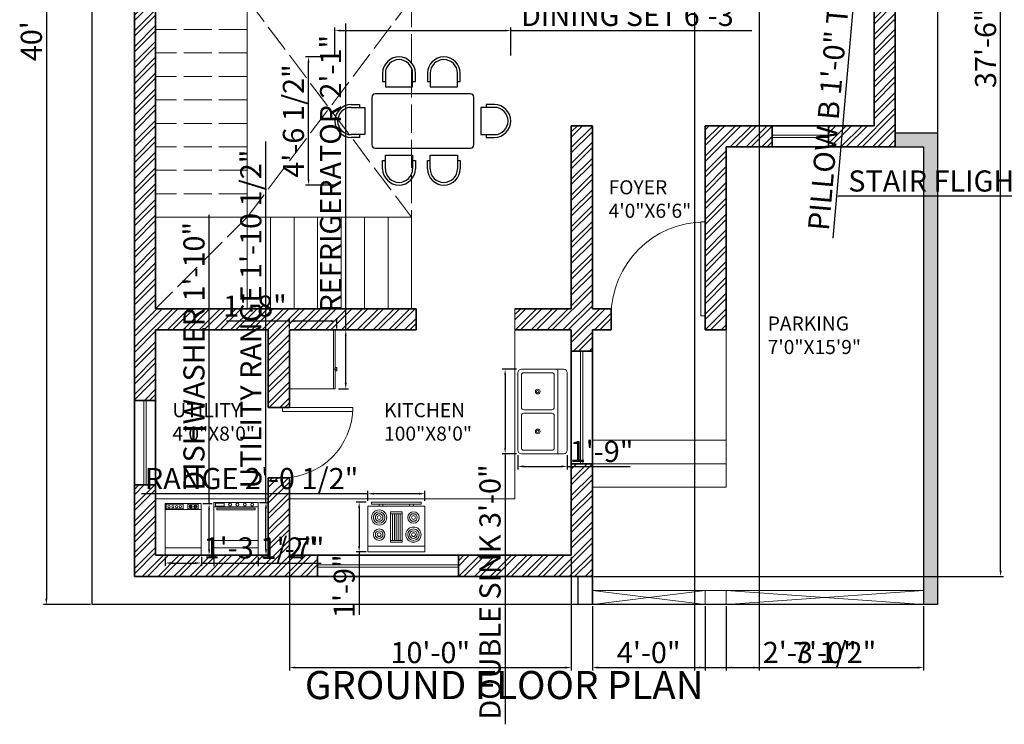
# Model space of a CAD drawing. Units: inches. Extents: x 638 to 1853, y 4393 to 5041.
# Tile 1 of 6: x 653 to 1072, y 4393 to 4693. Entities that reach past the tile are written whole.
import ezdxf

# ---------------------------------------------------------------- set-up
doc = ezdxf.new("R2010")
doc.units = ezdxf.units.IN
doc.linetypes.add('ACAD_ISO02W100', pattern=[15, 12, -3])
for name, color, linetype, lineweight in [('A-ANNO-DIMS', 2, 'Continuous', 18), ('A-ANNO-TEXT', 7, 'Continuous', 25), ('A-AREA-IDEN', 7, 'Continuous', 18), ('A-DOOR', 4, 'Continuous', 18), ('A-EQPM', 8, 'Continuous', 18), ('A-FLOR-CASE', 7, 'Continuous', 18), ('A-FLOR-FIXT', 9, 'Continuous', 18), ('A-FLOR-STRS', 7, 'Continuous', 18), ('A-FLOR-STRS-HIDN', 7, 'ACAD_ISO02W100', 18), ('A-FURN', 26, 'Continuous', 13), ('A-GLAZ', 5, 'Continuous', 18), ('A-WALL', 7, 'Continuous', 35), ('A-WALL-PATT', 251, 'Continuous', 13), ('A-WALL-PRPT', 7, 'Continuous', 25), ('A-WALL-PRPT-PATT', 141, 'Continuous', 13), ('C-PROP', 7, 'Continuous', 25), ('L-GATE', 3, 'Continuous', 18)]:
    doc.layers.add(name, color=color, linetype=linetype, lineweight=lineweight)
doc.layers.add('NOI THAT', color=42, linetype='Continuous')
doc.styles.get("Standard").update_dxf_attribs({"font": 'arial.ttf'})
doc.dimstyles.new('ISO-25', dxfattribs={"dimtxt": 9, "dimasz": 2.5, "dimexe": 1.25, "dimexo": 0.625, "dimtad": 1, "dimdec": 1, "dimlunit": 3, "dimtxsty": 'Standard', "dimcen": 2.5, "dimadec": 0, "dimazin": 0, "dimtfac": 1, "dimtdec": 1, "dimtmove": 0, "dimatfit": 3, "dimfxl": 1, "dimarcsym": 0})

# ---------------------------------------------------------------- blocks, each defined once
blk = doc.blocks.new('*U5')
for p, q in [((0, 0), (0, -6)), ((-40, 0), (-40, -6))]:
    blk.add_line(p, q)
blk.add_lwpolyline([(0, 0), (0, 40), (-1.75, 40), (-1.75, 0)], close=True)
blk.add_arc((0, 0), 40, 90, 180)
blk = doc.blocks.new('*U6')
for p, q in [((-30, 0), (-30, 6)), ((0, 0), (0, 6))]:
    blk.add_line(p, q)
blk.add_lwpolyline([(0, 0), (0, -30), (-1.75, -30), (-1.75, 0)], close=True)
blk.add_arc((0, 0), 30, 180, 270)
blk = doc.blocks.new('*D17')
at = {"layer": 'A-ANNO-DIMS', "color": 0, "lineweight": -2, "transparency": 16777216}
for p, q in [((682.72, 4924.19), (662.61, 4924.19)), ((663.86, 4921.69), (663.86, 4446.69)), ((682.72, 4444.19), (662.61, 4444.19))]:
    blk.add_line(p, q, dxfattribs=at)
at = {"layer": 'A-ANNO-DIMS', "color": 0, "transparency": 16777216}
for points in [[(663.44, 4921.69), (664.28, 4921.69), (663.86, 4924.19)], [(663.44, 4446.69), (664.28, 4446.69), (663.86, 4444.19)]]:
    blk.add_solid(points, dxfattribs=at)
at = {"layer": 'Defpoints', "color": 0, "transparency": 16777216}
for p in [(683.34, 4924.19), (663.86, 4444.19), (683.34, 4444.19)]:
    blk.add_point(p, dxfattribs=at)
at = {"layer": 'A-ANNO-DIMS', "color": 0, "transparency": 16777216, "insert": (658.64, 4684.19), "char_height": 9, "attachment_point": 5, "rotation": 90}
blk.add_mtext("40'", dxfattribs=at)
blk = doc.blocks.new('A$C3F0C2877')
at = {"layer": 'NOI THAT'}
for p, q in [((700, 1640), (700, 1520)), ((740, 1640), (740, 1440)), ((1140, 1440), (1140, 1640)), ((1180, 1520), (1180, 1640)), ((1358, 1640), (1358, 1520)), ((1398, 1640), (1398, 1440)), ((1798, 1440), (1798, 1640)), ((1838, 1520), (1838, 1640)), ((700, 1520), (740, 1520)), ((1140, 1520), (1180, 1520)), ((1358, 1520), (1398, 1520)), ((1798, 1520), (1838, 1520)), ((1988, 1340), (590, 1340)), ((740, 1440), (1140, 1440)), ((1398, 1440), (1798, 1440)), ((240, 1180), (360, 1180)), ((360, 1180), (360, 1140)), ((540, 1290), (540, 590)), ((2038, 590), (2038, 1290)), ((2339, 1180), (2219, 1180)), ((2219, 1180), (2219, 1140)), ((240, 1140), (440, 1140)), ((440, 1140), (440, 740)), ((2139, 1140), (2139, 740)), ((2339, 1140), (2139, 1140)), ((440, 740), (240, 740)), ((360, 740), (360, 700)), ((2139, 740), (2339, 740)), ((2219, 740), (2219, 700)), ((360, 700), (240, 700)), ((2219, 700), (2339, 700)), ((590, 540), (1988, 540)), ((740, 440), (1140, 440)), ((740, 240), (740, 440)), ((1140, 440), (1140, 240)), ((1398, 440), (1798, 440)), ((1398, 240), (1398, 440)), ((1798, 440), (1798, 240)), ((700, 360), (740, 360)), ((700, 240), (700, 360)), ((1140, 360), (1180, 360)), ((1180, 360), (1180, 240)), ((1358, 360), (1398, 360)), ((1358, 240), (1358, 360)), ((1798, 360), (1838, 360)), ((1838, 360), (1838, 240))]:
    blk.add_line(p, q, dxfattribs=at)
for centre, radius, start, end in [((940, 1640), 240, 0, 180), ((1598, 1640), 240, 0, 180), ((940, 1640), 200, 0, 180), ((1598, 1640), 200, 0, 180), ((590, 1290), 50, 90, 180), ((1988, 1290), 50, 0, 90), ((240, 940), 240, 90, 270), ((2339, 940), 240, 270, 90), ((240, 940), 200, 90, 270), ((2339, 940), 200, 270, 90), ((590, 590), 50, 180, 270), ((1988, 590), 50, 270, 0), ((940, 240), 240, 180, 0), ((940, 240), 200, 180, 0), ((1598, 240), 240, 180, 0), ((1598, 240), 200, 180, 0)]:
    blk.add_arc(centre, radius, start, end, dxfattribs=at)
blk = doc.blocks.new('Sink-double - 36 in top')
for p, q in [((-18, -4), (18, -4)), ((-0.75, -18.5), (-0.75, -6.5)), ((0.75, -6.5), (0.75, -18.5))]:
    blk.add_line(p, q)
for points in [[(-16.5, 0), (16.5, 0)], [(-18, -19.5), (-18, -1.5)], [(18, -1.5), (18, -19.5)], [(-16.5, -18.5), (-16.5, -6.5)], [(-15.5, -5.5), (-1.75, -5.5)], [(1.75, -5.5), (15.5, -5.5)], [(16.5, -6.5), (16.5, -18.5)], [(-1.75, -19.5), (-15.5, -19.5)], [(15.5, -19.5), (1.75, -19.5)], [(16.5, -21), (-16.5, -21)]]:
    blk.add_lwpolyline(points)
for centre, radius in [((-8.5, -12.5), 1), ((-8.5, -12.5), 0.5), ((8.5, -12.5), 1), ((8.5, -12.5), 0.5)]:
    blk.add_circle(centre, radius)
for centre, radius, start, end in [((-16.5, -1.5), 1.5, 90, 180), ((16.5, -1.5), 1.5, 0, 90), ((-15.5, -6.5), 1, 90, 180), ((-1.75, -6.5), 1, 0, 90), ((1.75, -6.5), 1, 90, 180), ((15.5, -6.5), 1, 0, 90), ((-16.5, -19.5), 1.5, 180, 270), ((-15.5, -18.5), 1, 180, 270), ((-1.75, -18.5), 1, 270, 0), ((1.75, -18.5), 1, 180, 270), ((15.5, -18.5), 1, 270, 0), ((16.5, -19.5), 1.5, 270, 0)]:
    blk.add_arc(centre, radius, start, end)
blk = doc.blocks.new('Range-Oven - 30 in top')
for p, q in [((0, -3), (30, -3)), ((12, -6), (18, -6)), ((13, -20), (13, -6)), ((14, -6), (14, -20)), ((15, -20), (15, -6)), ((16, -6), (16, -20)), ((17, -20), (17, -6)), ((18, -20), (12, -20)), ((6, -24), (6, -25)), ((8, -25), (8, -24)), ((22, -25), (22, -24)), ((24, -24), (24, -25))]:
    blk.add_line(p, q)
for points in [[(0, -24), (0, 0), (30, 0), (30, -24)], [(12, -21), (12, -5), (18, -5), (18, -21)], [(2, -26), (2, -25), (28, -25), (28, -26)]]:
    blk.add_lwpolyline(points, close=True)
for centre, radius in [((6, -9), 4), ((6, -9), 3), ((6, -9), 2), ((6, -9), 1), ((24, -9), 3), ((24, -9), 2), ((24, -9), 1), ((6, -18), 3), ((24, -18), 4), ((24, -18), 3), ((6, -18), 2), ((6, -18), 1), ((24, -18), 2), ((24, -18), 1)]:
    blk.add_circle(centre, radius)
blk = doc.blocks.new('Range-Oven - 30 in front')
for p, q in [((0, 33.00005), (30, 33.00005)), ((30, 10), (0, 10)), ((0, 5), (30, 5))]:
    blk.add_line(p, q)
for points in [[(0, 0), (0, 36.00005), (30, 36.00005), (30, 0)], [(1, 33.50005), (1, 35.50005), (7, 35.50005), (7, 33.50005)], [(2, 31.00005), (2, 32.00005), (28, 32.00005), (28, 31.00005)]]:
    blk.add_lwpolyline(points, close=True)
for centre in [(11, 34.50005), (16, 34.50005), (21, 34.50005), (26, 34.50005)]:
    blk.add_circle(centre, 1)
blk = doc.blocks.new('Dishwasher')
for p, q in [((16.3156, 33.1843), (16.5, 33)), ((17, 32.75), (17, 33.5)), ((17.5, 33), (17.6938, 33.1938)), ((19.3156, 33.1843), (19.5, 33)), ((20, 32.75), (20, 33.5)), ((20.5, 33), (20.6938, 33.1938)), ((24, 30.5), (0, 30.5)), ((16, 32.5), (16.75, 32.5)), ((16.5, 32), (16.2942, 31.7942)), ((17, 32.25), (17, 31.5)), ((18, 32.5), (17.25, 32.5)), ((17.7061, 31.7939), (17.5, 32)), ((19, 32.5), (19.75, 32.5)), ((19.5, 32), (19.2942, 31.7942)), ((20, 32.25), (20, 31.5)), ((21, 32.5), (20.25, 32.5)), ((20.7061, 31.7939), (20.5, 32)), ((0, 5), (24, 5))]:
    blk.add_line(p, q)
for points in [[(0, 0), (0, 34.5), (24, 34.5), (24, 0)], [(0.5, 31), (0.5, 34), (12, 34), (12, 31)], [(15, 31), (15, 34), (22, 34), (22, 31)]]:
    blk.add_lwpolyline(points, close=True)
for centre, radius in [((2.5, 32.5), 0.75), ((5, 32.5), 0.75), ((7.5, 32.5), 0.75), ((10, 32.5), 0.75), ((17, 32.5), 1), ((20, 32.5), 1)]:
    blk.add_circle(centre, radius)
blk = doc.blocks.new('Refrigerator-2 door - 36 in top')
for p, q in [((0, -26.999999), (36, -26.999999)), ((11, -27.999999), (11, -28.999999)), ((11, -28.999999), (13, -28.999999)), ((12, -26.999999), (12, -28.999999)), ((13, -28.999999), (13, -27.999999))]:
    blk.add_line(p, q)
blk.add_lwpolyline([(0, -27.999999), (0, 0), (36, 0), (36, -27.999999)], close=True)
blk = doc.blocks.new('WINDOW-GLAZING-24IN')
for p, q in [((0, 24), (0, 0)), ((1, 24), (1, 0))]:
    blk.add_line(p, q)
blk = doc.blocks.new('STAIR-WELL-OPENING')
for p, q in [((0, 93), (70, 0)), ((0, 0), (70, 93))]:
    blk.add_line(p, q)
blk.add_lwpolyline([(0, 93), (70, 93), (70, 0), (0, 0)], close=True)
blk = doc.blocks.new('STAIR-RUN-7-TREAD')
for p, q in [((0, 0), (0, 39)), ((10, 0), (10, 39)), ((20, 0), (20, 39)), ((30, 0), (30, 39)), ((40, 0), (40, 39)), ((50, 0), (50, 39)), ((60, 0), (60, 39))]:
    blk.add_line(p, q)
blk = doc.blocks.new('*D50')
at = {"layer": 'A-ANNO-DIMS', "color": 0, "lineweight": -2, "transparency": 16777216}
for p, q in [((1009.16, 4733.11), (1011.59, 4732.9)), ((1010.13, 4730.52), (1009.51, 4723.42)), ((1009.29, 4720.93), (998.74, 4600.35)), ((1008.1, 4721.03), (1010.54, 4720.82))]:
    blk.add_line(p, q, dxfattribs=at)
at = {"layer": 'A-ANNO-DIMS', "color": 0, "transparency": 16777216}
for points in [[(1009.71, 4730.55), (1010.54, 4730.48), (1010.35, 4733.01)], [(1009.09, 4723.46), (1009.92, 4723.38), (1009.29, 4720.93)]]:
    blk.add_solid(points, dxfattribs=at)
at = {"layer": 'Defpoints', "color": 0, "transparency": 16777216}
for p in [(1008.54, 4733.16), (1007.48, 4721.09), (1009.29, 4720.93)]:
    blk.add_point(p, dxfattribs=at)
at = {"layer": 'A-ANNO-DIMS', "color": 0, "transparency": 16777216, "insert": (998.65, 4659.85), "char_height": 9, "attachment_point": 5, "rotation": 85}
blk.add_mtext('PILLOW B 1\'-0" TYP.', dxfattribs=at)
blk = doc.blocks.new('*D58')
at = {"layer": 'A-ANNO-DIMS', "color": 0, "lineweight": -2, "transparency": 16777216}
for p, q in [((1148.08, 4618.19), (1000.8, 4618.19)), ((1148.08, 4609.82), (1148.08, 4619.44)), ((1205.58, 4618.19), (1150.58, 4618.19)), ((1208.08, 4609.82), (1208.08, 4619.44))]:
    blk.add_line(p, q, dxfattribs=at)
at = {"layer": 'A-ANNO-DIMS', "color": 0, "transparency": 16777216}
for points in [[(1150.58, 4618.61), (1150.58, 4617.78), (1148.08, 4618.19)], [(1205.58, 4618.61), (1205.58, 4617.78), (1208.08, 4618.19)]]:
    blk.add_solid(points, dxfattribs=at)
at = {"layer": 'Defpoints', "color": 0, "transparency": 16777216}
for p in [(1148.08, 4618.19), (1148.08, 4609.19), (1208.08, 4609.19)]:
    blk.add_point(p, dxfattribs=at)
at = {"layer": 'A-ANNO-DIMS', "color": 0, "transparency": 16777216, "insert": (1073.19, 4623.47), "char_height": 9, "attachment_point": 5}
blk.add_mtext('STAIR FLIGHT 5\'-0" TYP.', dxfattribs=at)
blk = doc.blocks.new('*D62')
at = {"layer": 'A-ANNO-DIMS', "color": 0, "lineweight": -2, "transparency": 16777216}
for p, q in [((786.73, 4678.11), (786.73, 4689.96)), ((789.23, 4688.71), (859.1, 4688.71)), ((861.6, 4678.11), (861.6, 4689.96)), ((861.6, 4688.71), (964.27, 4688.71))]:
    blk.add_line(p, q, dxfattribs=at)
at = {"layer": 'A-ANNO-DIMS', "color": 0, "transparency": 16777216}
for points in [[(789.23, 4689.13), (789.23, 4688.3), (786.73, 4688.71)], [(859.1, 4689.13), (859.1, 4688.3), (861.6, 4688.71)]]:
    blk.add_solid(points, dxfattribs=at)
at = {"layer": 'Defpoints', "color": 0, "transparency": 16777216}
for p in [(861.6, 4688.71), (786.73, 4677.48), (861.6, 4677.48)]:
    blk.add_point(p, dxfattribs=at)
at = {"layer": 'A-ANNO-DIMS', "color": 0, "transparency": 16777216, "insert": (914.18, 4694), "char_height": 9, "attachment_point": 5}
blk.add_mtext('DINING SET 6\'-3"', dxfattribs=at)
blk = doc.blocks.new('*D63')
at = {"layer": 'A-ANNO-DIMS', "color": 0, "lineweight": -2, "transparency": 16777216}
for p, q in [((786.11, 4677.48), (774.25, 4677.48)), ((775.5, 4625.4), (775.5, 4674.98)), ((786.11, 4622.9), (774.25, 4622.9))]:
    blk.add_line(p, q, dxfattribs=at)
at = {"layer": 'A-ANNO-DIMS', "color": 0, "transparency": 16777216}
for points in [[(775.08, 4674.98), (775.92, 4674.98), (775.5, 4677.48)], [(775.08, 4625.4), (775.92, 4625.4), (775.5, 4622.9)]]:
    blk.add_solid(points, dxfattribs=at)
at = {"layer": 'Defpoints', "color": 0, "transparency": 16777216}
for p in [(775.5, 4677.48), (786.73, 4677.48), (786.73, 4622.9)]:
    blk.add_point(p, dxfattribs=at)
at = {"layer": 'A-ANNO-DIMS', "color": 0, "transparency": 16777216, "insert": (770.22, 4650.19), "char_height": 9, "attachment_point": 5, "rotation": 90}
blk.add_mtext('4\'-6 1/2"', dxfattribs=at)
blk = doc.blocks.new('*D64')
at = {"layer": 'A-ANNO-DIMS', "color": 0, "lineweight": -2, "transparency": 16777216}
for p, q in [((863.99, 4544.45), (857.97, 4544.45)), ((859.22, 4541.95), (859.22, 4510.95)), ((863.99, 4508.45), (857.97, 4508.45)), ((859.22, 4508.45), (859.22, 4393.19))]:
    blk.add_line(p, q, dxfattribs=at)
at = {"layer": 'A-ANNO-DIMS', "color": 0, "transparency": 16777216}
for points in [[(858.8, 4541.95), (859.63, 4541.95), (859.22, 4544.45)], [(858.8, 4510.95), (859.63, 4510.95), (859.22, 4508.45)]]:
    blk.add_solid(points, dxfattribs=at)
at = {"layer": 'Defpoints', "color": 0, "transparency": 16777216}
for p in [(864.62, 4544.45), (859.22, 4508.45), (864.62, 4508.45)]:
    blk.add_point(p, dxfattribs=at)
at = {"layer": 'A-ANNO-DIMS', "color": 0, "transparency": 16777216, "insert": (853.93, 4449.57), "char_height": 9, "attachment_point": 5, "rotation": 90}
blk.add_mtext('DOUBLE SINK 3\'-0"', dxfattribs=at)
blk = doc.blocks.new('*D65')
at = {"layer": 'A-ANNO-DIMS', "color": 0, "lineweight": -2, "transparency": 16777216}
for p, q in [((864.62, 4507.83), (864.62, 4501.8)), ((885.62, 4507.83), (885.62, 4501.8)), ((867.12, 4503.05), (883.12, 4503.05)), ((885.62, 4503.05), (912.45, 4503.05))]:
    blk.add_line(p, q, dxfattribs=at)
at = {"layer": 'A-ANNO-DIMS', "color": 0, "transparency": 16777216}
for points in [[(867.12, 4503.47), (867.12, 4502.64), (864.62, 4503.05)], [(883.12, 4503.47), (883.12, 4502.64), (885.62, 4503.05)]]:
    blk.add_solid(points, dxfattribs=at)
at = {"layer": 'Defpoints', "color": 0, "transparency": 16777216}
for p in [(864.62, 4508.45), (885.62, 4508.45), (885.62, 4503.05)]:
    blk.add_point(p, dxfattribs=at)
at = {"layer": 'A-ANNO-DIMS', "color": 0, "transparency": 16777216, "insert": (900.28, 4508.27), "char_height": 9, "attachment_point": 5}
blk.add_mtext('1\'-9"', dxfattribs=at)
blk = doc.blocks.new('*D66')
at = {"layer": 'A-ANNO-DIMS', "color": 0, "lineweight": -2, "transparency": 16777216}
for p, q in [((800.7, 4491.43), (704.32, 4491.43)), ((800.7, 4488.41), (800.7, 4492.68)), ((822.53, 4491.43), (803.2, 4491.43)), ((825.03, 4488.41), (825.03, 4492.68))]:
    blk.add_line(p, q, dxfattribs=at)
at = {"layer": 'A-ANNO-DIMS', "color": 0, "transparency": 16777216}
for points in [[(803.2, 4491.85), (803.2, 4491.01), (800.7, 4491.43)], [(822.53, 4491.85), (822.53, 4491.01), (825.03, 4491.43)]]:
    blk.add_solid(points, dxfattribs=at)
at = {"layer": 'Defpoints', "color": 0, "transparency": 16777216}
for p in [(800.7, 4491.43), (800.7, 4487.78), (825.03, 4487.78)]:
    blk.add_point(p, dxfattribs=at)
at = {"layer": 'A-ANNO-DIMS', "color": 0, "transparency": 16777216, "insert": (751.26, 4496.71), "char_height": 9, "attachment_point": 5}
blk.add_mtext('RANGE 2\'-0 1/2"', dxfattribs=at)
blk = doc.blocks.new('*D67')
at = {"layer": 'A-ANNO-DIMS', "color": 0, "lineweight": -2, "transparency": 16777216}
for p, q in [((800.07, 4487.78), (795.8, 4487.78)), ((797.05, 4485.28), (797.05, 4469.19)), ((800.07, 4466.69), (795.8, 4466.69)), ((797.05, 4466.69), (797.05, 4439.87))]:
    blk.add_line(p, q, dxfattribs=at)
at = {"layer": 'A-ANNO-DIMS', "color": 0, "transparency": 16777216}
for points in [[(796.63, 4485.28), (797.47, 4485.28), (797.05, 4487.78)], [(796.63, 4469.19), (797.47, 4469.19), (797.05, 4466.69)]]:
    blk.add_solid(points, dxfattribs=at)
at = {"layer": 'Defpoints', "color": 0, "transparency": 16777216}
for p in [(800.7, 4487.78), (797.05, 4466.69), (800.7, 4466.69)]:
    blk.add_point(p, dxfattribs=at)
at = {"layer": 'A-ANNO-DIMS', "color": 0, "transparency": 16777216, "insert": (791.83, 4452.03), "char_height": 9, "attachment_point": 5, "rotation": 90}
blk.add_mtext('1\'-9"', dxfattribs=at)
blk = doc.blocks.new('*D68')
at = {"layer": 'A-ANNO-DIMS', "color": 0, "lineweight": -2, "transparency": 16777216}
for p, q in [((757.38, 4487.74), (757.38, 4641.41)), ((754.62, 4487.74), (758.63, 4487.74)), ((757.38, 4467.69), (757.38, 4485.24)), ((754.62, 4465.19), (758.63, 4465.19))]:
    blk.add_line(p, q, dxfattribs=at)
at = {"layer": 'A-ANNO-DIMS', "color": 0, "transparency": 16777216}
for points in [[(756.96, 4485.24), (757.8, 4485.24), (757.38, 4487.74)], [(756.96, 4467.69), (757.8, 4467.69), (757.38, 4465.19)]]:
    blk.add_solid(points, dxfattribs=at)
at = {"layer": 'Defpoints', "color": 0, "transparency": 16777216}
for p in [(754, 4487.74), (757.38, 4487.74), (754, 4465.19)]:
    blk.add_point(p, dxfattribs=at)
at = {"layer": 'A-ANNO-DIMS', "color": 0, "transparency": 16777216, "insert": (752.1, 4565.82), "char_height": 9, "attachment_point": 5, "rotation": 90}
blk.add_mtext('UTILITY RANGE 1\'-10 1/2"', dxfattribs=at)
blk = doc.blocks.new('*D69')
at = {"layer": 'A-ANNO-DIMS', "color": 0, "lineweight": -2, "transparency": 16777216}
for p, q in [((735.21, 4464.57), (735.21, 4460.56)), ((737.71, 4461.81), (751.5, 4461.81)), ((754, 4464.57), (754, 4460.56)), ((754, 4461.81), (780.82, 4461.81))]:
    blk.add_line(p, q, dxfattribs=at)
at = {"layer": 'A-ANNO-DIMS', "color": 0, "transparency": 16777216}
for points in [[(737.71, 4462.23), (737.71, 4461.4), (735.21, 4461.81)], [(751.5, 4462.23), (751.5, 4461.4), (754, 4461.81)]]:
    blk.add_solid(points, dxfattribs=at)
at = {"layer": 'Defpoints', "color": 0, "transparency": 16777216}
for p in [(735.21, 4465.19), (754, 4465.19), (754, 4461.81)]:
    blk.add_point(p, dxfattribs=at)
at = {"layer": 'A-ANNO-DIMS', "color": 0, "transparency": 16777216, "insert": (768.66, 4466.96), "char_height": 9, "attachment_point": 5}
blk.add_mtext('1\'-7"', dxfattribs=at)
blk = doc.blocks.new('*D70')
at = {"layer": 'A-ANNO-DIMS', "color": 0, "lineweight": -2, "transparency": 16777216}
for p, q in [((733.16, 4487.24), (733.16, 4610.17)), ((730.48, 4487.24), (734.41, 4487.24)), ((733.16, 4467.69), (733.16, 4484.74)), ((730.48, 4465.19), (734.41, 4465.19))]:
    blk.add_line(p, q, dxfattribs=at)
at = {"layer": 'A-ANNO-DIMS', "color": 0, "transparency": 16777216}
for points in [[(732.74, 4484.74), (733.57, 4484.74), (733.16, 4487.24)], [(732.74, 4467.69), (733.57, 4467.69), (733.16, 4465.19)]]:
    blk.add_solid(points, dxfattribs=at)
at = {"layer": 'Defpoints', "color": 0, "transparency": 16777216}
for p in [(729.85, 4487.24), (733.16, 4487.24), (729.85, 4465.19)]:
    blk.add_point(p, dxfattribs=at)
at = {"layer": 'A-ANNO-DIMS', "color": 0, "transparency": 16777216, "insert": (727.88, 4549.96), "char_height": 9, "attachment_point": 5, "rotation": 90}
blk.add_mtext('DISHWASHER 1\'-10"', dxfattribs=at)
blk = doc.blocks.new('*D71')
at = {"layer": 'A-ANNO-DIMS', "color": 0, "lineweight": -2, "transparency": 16777216}
for p, q in [((714.51, 4464.57), (714.51, 4460.64)), ((717.01, 4461.89), (727.35, 4461.89)), ((729.85, 4464.57), (729.85, 4460.64)), ((729.85, 4461.89), (777.65, 4461.89))]:
    blk.add_line(p, q, dxfattribs=at)
at = {"layer": 'A-ANNO-DIMS', "color": 0, "transparency": 16777216}
for points in [[(717.01, 4462.3), (717.01, 4461.47), (714.51, 4461.89)], [(727.35, 4462.3), (727.35, 4461.47), (729.85, 4461.89)]]:
    blk.add_solid(points, dxfattribs=at)
at = {"layer": 'Defpoints', "color": 0, "transparency": 16777216}
for p in [(714.51, 4465.19), (729.85, 4465.19), (729.85, 4461.89)]:
    blk.add_point(p, dxfattribs=at)
at = {"layer": 'A-ANNO-DIMS', "color": 0, "transparency": 16777216, "insert": (755, 4467.17), "char_height": 9, "attachment_point": 5}
blk.add_mtext('1\'-3 1/2"', dxfattribs=at)
blk = doc.blocks.new('*D72')
at = {"layer": 'A-ANNO-DIMS', "color": 0, "lineweight": -2, "transparency": 16777216}
for p, q in [((791.33, 4561.19), (791.33, 4691.79)), ((788.19, 4561.19), (792.58, 4561.19)), ((791.33, 4538.59), (791.33, 4558.69)), ((788.19, 4536.09), (792.58, 4536.09))]:
    blk.add_line(p, q, dxfattribs=at)
at = {"layer": 'A-ANNO-DIMS', "color": 0, "transparency": 16777216}
for points in [[(790.91, 4558.69), (791.74, 4558.69), (791.33, 4561.19)], [(790.91, 4538.59), (791.74, 4538.59), (791.33, 4536.09)]]:
    blk.add_solid(points, dxfattribs=at)
at = {"layer": 'Defpoints', "color": 0, "transparency": 16777216}
for p in [(787.56, 4561.19), (791.33, 4561.19), (787.56, 4536.09)]:
    blk.add_point(p, dxfattribs=at)
at = {"layer": 'A-ANNO-DIMS', "color": 0, "transparency": 16777216, "insert": (786.05, 4627.74), "char_height": 9, "attachment_point": 5, "rotation": 90}
blk.add_mtext('REFRIGERATOR 2\'-1"', dxfattribs=at)
blk = doc.blocks.new('*D73')
at = {"layer": 'A-ANNO-DIMS', "color": 0, "lineweight": -2, "transparency": 16777216}
for p, q in [((767.34, 4561.82), (767.34, 4566.21)), ((787.56, 4561.82), (787.56, 4566.21)), ((767.34, 4564.96), (740.51, 4564.96)), ((785.06, 4564.96), (769.84, 4564.96))]:
    blk.add_line(p, q, dxfattribs=at)
at = {"layer": 'A-ANNO-DIMS', "color": 0, "transparency": 16777216}
for points in [[(769.84, 4565.38), (769.84, 4564.54), (767.34, 4564.96)], [(785.06, 4565.38), (785.06, 4564.54), (787.56, 4564.96)]]:
    blk.add_solid(points, dxfattribs=at)
at = {"layer": 'Defpoints', "color": 0, "transparency": 16777216}
for p in [(767.34, 4564.96), (767.34, 4561.19), (787.56, 4561.19)]:
    blk.add_point(p, dxfattribs=at)
at = {"layer": 'A-ANNO-DIMS', "color": 0, "transparency": 16777216, "insert": (752.68, 4570.18), "char_height": 9, "attachment_point": 5}
blk.add_mtext('1\'-8"', dxfattribs=at)
blk = doc.blocks.new('*D75')
at = {"layer": 'A-ANNO-DIMS', "color": 0, "lineweight": -2, "transparency": 16777216}
for p, q in [((1025.97, 4906.19), (1071.42, 4906.19)), ((1070.17, 4458.69), (1070.17, 4903.69)), ((896.97, 4456.19), (1071.42, 4456.19))]:
    blk.add_line(p, q, dxfattribs=at)
at = {"layer": 'A-ANNO-DIMS', "color": 0, "transparency": 16777216}
for points in [[(1069.75, 4903.69), (1070.58, 4903.69), (1070.17, 4906.19)], [(1069.75, 4458.69), (1070.58, 4458.69), (1070.17, 4456.19)]]:
    blk.add_solid(points, dxfattribs=at)
at = {"layer": 'Defpoints', "color": 0, "transparency": 16777216}
for p in [(1025.34, 4906.19), (1070.17, 4906.19), (896.34, 4456.19)]:
    blk.add_point(p, dxfattribs=at)
at = {"layer": 'A-ANNO-DIMS', "color": 0, "transparency": 16777216, "insert": (1064.94, 4681.19), "char_height": 9, "attachment_point": 5, "rotation": 90}
blk.add_mtext('37\'-6"', dxfattribs=at)
blk = doc.blocks.new('*D78')
at = {"layer": 'A-ANNO-DIMS', "color": 0, "lineweight": -2, "transparency": 16777216}
for p, q in [((953.34, 4443.57), (953.34, 4416.12)), ((1037.34, 4443.57), (1037.34, 4416.12)), ((955.84, 4417.37), (1034.84, 4417.37))]:
    blk.add_line(p, q, dxfattribs=at)
at = {"layer": 'A-ANNO-DIMS', "color": 0, "transparency": 16777216}
for points in [[(955.84, 4417.79), (955.84, 4416.95), (953.34, 4417.37)], [(1034.84, 4417.79), (1034.84, 4416.95), (1037.34, 4417.37)]]:
    blk.add_solid(points, dxfattribs=at)
at = {"layer": 'Defpoints', "color": 0, "transparency": 16777216}
for p in [(953.34, 4444.19), (1037.34, 4444.19), (1037.34, 4417.37)]:
    blk.add_point(p, dxfattribs=at)
at = {"layer": 'A-ANNO-DIMS', "color": 0, "transparency": 16777216, "insert": (995.34, 4422.59), "char_height": 9, "attachment_point": 5}
blk.add_mtext('7\'-0"', dxfattribs=at)
blk = doc.blocks.new('*D79')
at = {"layer": 'A-ANNO-DIMS', "color": 0, "lineweight": -2, "transparency": 16777216}
for p, q in [((896.34, 4443.57), (896.34, 4416.12)), ((944.34, 4443.57), (944.34, 4416.12)), ((898.84, 4417.37), (941.84, 4417.37))]:
    blk.add_line(p, q, dxfattribs=at)
at = {"layer": 'A-ANNO-DIMS', "color": 0, "transparency": 16777216}
for points in [[(898.84, 4417.79), (898.84, 4416.95), (896.34, 4417.37)], [(941.84, 4417.79), (941.84, 4416.95), (944.34, 4417.37)]]:
    blk.add_solid(points, dxfattribs=at)
at = {"layer": 'Defpoints', "color": 0, "transparency": 16777216}
for p in [(896.34, 4444.19), (944.34, 4444.19), (944.34, 4417.37)]:
    blk.add_point(p, dxfattribs=at)
at = {"layer": 'A-ANNO-DIMS', "color": 0, "transparency": 16777216, "insert": (920.34, 4422.59), "char_height": 9, "attachment_point": 5}
blk.add_mtext('4\'-0"', dxfattribs=at)
blk = doc.blocks.new('*D81')
at = {"layer": 'A-ANNO-DIMS', "color": 0, "lineweight": -2, "transparency": 16777216}
for p, q in [((767.34, 4464.57), (767.34, 4416.12)), ((887.34, 4464.57), (887.34, 4416.12)), ((769.84, 4417.37), (884.84, 4417.37))]:
    blk.add_line(p, q, dxfattribs=at)
at = {"layer": 'A-ANNO-DIMS', "color": 0, "transparency": 16777216}
for points in [[(769.84, 4417.79), (769.84, 4416.95), (767.34, 4417.37)], [(884.84, 4417.79), (884.84, 4416.95), (887.34, 4417.37)]]:
    blk.add_solid(points, dxfattribs=at)
at = {"layer": 'Defpoints', "color": 0, "transparency": 16777216}
for p in [(767.34, 4465.19), (887.34, 4465.19), (887.34, 4417.37)]:
    blk.add_point(p, dxfattribs=at)
at = {"layer": 'A-ANNO-DIMS', "color": 0, "transparency": 16777216, "insert": (827.34, 4422.59), "char_height": 9, "attachment_point": 5}
blk.add_mtext('10\'-0"', dxfattribs=at)
blk = doc.blocks.new('*D84')
at = {"layer": 'A-ANNO-DIMS', "color": 0, "lineweight": -2, "transparency": 16777216}
for p, q in [((939.87, 4743.42), (939.87, 4416.12)), ((967.43, 4743.42), (967.43, 4416.12)), ((942.37, 4417.37), (964.93, 4417.37)), ((967.43, 4417.37), (1016.23, 4417.37))]:
    blk.add_line(p, q, dxfattribs=at)
at = {"layer": 'A-ANNO-DIMS', "color": 0, "transparency": 16777216}
for points in [[(942.37, 4417.79), (942.37, 4416.95), (939.87, 4417.37)], [(964.93, 4417.79), (964.93, 4416.95), (967.43, 4417.37)]]:
    blk.add_solid(points, dxfattribs=at)
at = {"layer": 'Defpoints', "color": 0, "transparency": 16777216}
for p in [(939.87, 4744.04), (967.43, 4744.04), (967.43, 4417.37)]:
    blk.add_point(p, dxfattribs=at)
at = {"layer": 'A-ANNO-DIMS', "color": 0, "transparency": 16777216, "insert": (993.08, 4422.65), "char_height": 9, "attachment_point": 5}
blk.add_mtext('2\'-3 1/2"', dxfattribs=at)

msp = doc.modelspace()

# ---------------------------------------------------------------- hatches: boundary and pattern name
at = {"layer": 'A-WALL-PATT', "transparency": 33554687}
h = msp.add_hatch(dxfattribs=at)
h.set_pattern_fill('ANSI32', color=256, scale=0.5)
h.paths.add_polyline_path([(779.34, 4906.19), (701.34, 4906.19), (701.34, 4531.19), (710.34, 4531.19), (710.34, 4561.19), (758.34, 4561.19), (758.34, 4528.19), (764.34, 4528.19), (767.34, 4528.19), (767.34, 4561.19), (821.34, 4561.19), (821.34, 4570.19), (710.34, 4570.19), (710.34, 4756.19), (767.34, 4756.19), (767.34, 4702.19), (791.34, 4702.19), (791.34, 4708.19), (773.34, 4708.19), (773.34, 4756.19), (845.34, 4756.19), (845.34, 4708.19), (827.35, 4708.19), (827.35, 4705.02), (827.34, 4702.19), (851.34, 4702.19), (851.34, 4771.19), (845.34, 4771.19), (842.34, 4771.19), (842.34, 4765.19), (710.34, 4765.19), (710.34, 4897.19), (779.34, 4897.19)])
h.paths.add_polyline_path([(1025.34, 4906.19), (833.34, 4906.19), (833.34, 4897.19), (842.34, 4897.19), (842.34, 4882.21), (842.34, 4879.19), (851.34, 4879.19), (851.34, 4897.19), (914.34, 4897.19), (914.34, 4879.19), (920.34, 4879.19), (920.34, 4897.19), (1016.34, 4897.19), (1016.34, 4885.19), (1025.34, 4885.19)])
h.paths.add_polyline_path([(851.34, 4840.19), (1016.34, 4840.19), (1016.34, 4780.19), (1025.34, 4780.19), (1025.34, 4861.19), (1016.34, 4861.19), (1016.34, 4849.19), (842.34, 4849.19), (842.34, 4807.19), (851.34, 4807.19)])
h.paths.add_polyline_path([(1025.34, 4708.19), (1016.34, 4708.19), (1016.34, 4694.92), (1016.34, 4648.19), (996.84, 4648.19), (996.84, 4639.19), (1025.34, 4639.19)])
h.paths.add_polyline_path([(972.84, 4648.19), (944.34, 4648.19), (944.34, 4561.19), (953.34, 4561.19), (953.34, 4639.19), (972.84, 4639.19)])
h.paths.add_polyline_path([(896.34, 4648.19), (887.34, 4648.19), (887.34, 4570.19), (863.34, 4570.19), (863.34, 4561.19), (887.34, 4561.19), (887.34, 4552.19), (896.34, 4552.19), (896.34, 4561.19), (904.34, 4561.19), (904.34, 4567.19), (904.34, 4570.19), (896.34, 4570.19)])
h.paths.add_polyline_path([(896.34, 4504.19), (887.34, 4504.19), (887.34, 4465.19), (839.34, 4465.19), (839.34, 4456.19), (896.34, 4456.19)])
h.paths.add_polyline_path([(779.34, 4465.19), (767.34, 4465.19), (767.34, 4498.19), (758.34, 4498.19), (758.34, 4465.19), (710.34, 4465.19), (710.34, 4495.19), (701.34, 4495.19), (701.34, 4456.19), (779.34, 4456.19)])
h.paths.add_polyline_path([(865.86, 4868.68), (912.64, 4868.68), (912.64, 4891.07), (865.86, 4891.07)], flags=9)
h.paths.add_polyline_path([(730.31, 4828.82), (807.82, 4828.82), (807.82, 4851.21), (730.31, 4851.21)], flags=25)
at = {"layer": 'A-WALL-PRPT-PATT', "transparency": 33554687}
h = msp.add_hatch(color=256, dxfattribs=at)
h.dxf.hatch_style = 1
h.paths.add_polyline_path([(1043.34, 4645.19), (1025.34, 4645.19), (1025.34, 4639.19), (1037.34, 4639.19), (1037.34, 4444.19), (1043.34, 4444.19)])

# ---------------------------------------------------------------- linework, layer by layer
at = {"layer": 'A-FLOR-CASE'}
for p, q in [((863.34, 4489.19), (863.34, 4570.19)), ((758.34, 4489.19), (710.34, 4489.19)), ((863.34, 4489.19), (767.34, 4489.19))]:
    msp.add_line(p, q, dxfattribs=at)
at = {"layer": 'A-FLOR-STRS'}
for p, q in [((749.34, 4570.19), (749.34, 4719.19)), ((819.34, 4609.19), (710.34, 4609.19)), ((953.34, 4561.19), (953.34, 4494.19)), ((953.34, 4514.19), (896.34, 4514.19)), ((953.34, 4504.19), (896.34, 4504.19)), ((953.34, 4494.19), (896.34, 4494.19))]:
    msp.add_line(p, q, dxfattribs=at)
at = {"layer": 'A-FLOR-STRS-HIDN'}
for p, q in [((749.34, 4689.19), (710.34, 4689.19)), ((749.34, 4679.19), (710.34, 4679.19)), ((749.34, 4669.19), (710.34, 4669.19)), ((749.34, 4659.19), (710.34, 4659.19)), ((749.34, 4649.19), (710.34, 4649.19)), ((749.34, 4639.19), (710.34, 4639.19)), ((749.34, 4629.19), (710.34, 4629.19)), ((749.34, 4619.19), (710.34, 4619.19)), ((749.34, 4619.19), (710.34, 4619.19)), ((749.34, 4609.19), (710.34, 4570.19))]:
    msp.add_line(p, q, dxfattribs=at)
at = {"layer": 'A-GLAZ'}
for p, q in [((891.34, 4552.19), (891.34, 4504.19)), ((892.34, 4552.19), (892.34, 4504.19)), ((705.34, 4531.19), (705.34, 4495.19)), ((706.34, 4531.19), (706.34, 4495.19)), ((779.34, 4461.19), (839.34, 4461.19)), ((779.34, 4460.19), (839.34, 4460.19))]:
    msp.add_line(p, q, dxfattribs=at)
at = {"layer": 'A-WALL'}
for p, q in [((701.34, 4456.19), (701.34, 4906.19)), ((1025.34, 4906.19), (1025.34, 4639.19)), ((1016.34, 4840.19), (1016.34, 4648.19)), ((710.34, 4570.19), (710.34, 4756.19)), ((887.34, 4648.19), (896.34, 4648.19)), ((887.34, 4570.19), (887.34, 4648.19)), ((896.34, 4570.19), (896.34, 4648.19)), ((944.34, 4648.19), (1016.34, 4648.19)), ((944.34, 4561.19), (944.34, 4648.19)), ((972.84, 4639.19), (972.84, 4648.19)), ((996.84, 4639.19), (996.84, 4648.19)), ((953.34, 4639.19), (1025.34, 4639.19)), ((953.34, 4561.19), (953.34, 4639.19)), ((821.34, 4570.19), (710.34, 4570.19)), ((821.34, 4561.19), (821.34, 4570.19)), ((887.34, 4570.19), (863.34, 4570.19)), ((904.34, 4570.19), (896.34, 4570.19)), ((904.34, 4561.19), (904.34, 4570.19)), ((710.34, 4465.19), (710.34, 4561.19)), ((758.34, 4561.19), (710.34, 4561.19)), ((758.34, 4528.19), (758.34, 4561.19)), ((821.34, 4561.19), (767.34, 4561.19)), ((767.34, 4528.19), (767.34, 4561.19)), ((887.34, 4561.19), (863.34, 4561.19)), ((887.34, 4465.19), (887.34, 4561.19)), ((904.34, 4561.19), (896.34, 4561.19)), ((896.34, 4444.19), (896.34, 4561.19)), ((953.34, 4561.19), (944.34, 4561.19)), ((896.34, 4552.19), (887.34, 4552.19)), ((710.34, 4531.19), (701.34, 4531.19)), ((767.34, 4528.19), (758.34, 4528.19)), ((896.34, 4504.19), (887.34, 4504.19)), ((710.34, 4495.19), (701.34, 4495.19)), ((758.34, 4465.19), (758.34, 4498.19)), ((767.34, 4498.19), (758.34, 4498.19)), ((767.34, 4465.19), (767.34, 4498.19)), ((758.34, 4465.19), (710.34, 4465.19)), ((887.34, 4465.19), (767.34, 4465.19)), ((779.34, 4456.19), (779.34, 4465.19)), ((839.34, 4456.19), (839.34, 4465.19)), ((896.34, 4456.19), (701.34, 4456.19))]:
    msp.add_line(p, q, dxfattribs=at)
at = {"layer": 'A-WALL-PRPT'}
for p, q in [((1025.34, 4645.19), (1043.34, 4645.19)), ((1025.34, 4639.19), (1037.34, 4639.19)), ((1037.34, 4639.19), (1037.34, 4444.19)), ((890.34, 4444.19), (890.34, 4456.19))]:
    msp.add_line(p, q, dxfattribs=at)
at = {"layer": 'C-PROP'}
msp.add_lwpolyline([(683.34, 4924.19), (1043.34, 4924.19), (1043.34, 4444.19), (683.34, 4444.19)], close=True, dxfattribs=at)
at = {"layer": 'L-GATE'}
for p, q in [((896.34, 4444.19), (896.34, 4450.19)), ((896.34, 4450.19), (1037.34, 4450.19)), ((944.34, 4450.19), (896.34, 4444.19)), ((896.34, 4450.19), (944.34, 4444.19)), ((944.34, 4450.19), (944.34, 4444.19)), ((1037.34, 4450.19), (953.34, 4444.19)), ((953.34, 4450.19), (1037.34, 4444.19)), ((953.34, 4450.19), (953.34, 4444.19))]:
    msp.add_line(p, q, dxfattribs=at)

# ---------------------------------------------------------------- block references
at = {"layer": 'A-DOOR'}
msp.add_blockref('*U5', (944.34, 4567.19), dxfattribs=at)
at = {"layer": 'A-DOOR', "rotation": 89.99999999999999}
msp.add_blockref('*U6', (764.34, 4528.19), dxfattribs=at)
at = {"layer": 'A-EQPM'}
for name, p, xscale, yscale, zscale, rotation in [('Refrigerator-2 door - 36 in top', (767.34, 4536.09), 0.697290506458267, 0.697290506458267, 0.697290506458267, 90), ('Range-Oven - 30 in top', (825.03, 4466.69), 0.8110579885924902, 0.8110579885924902, 0.8110579885924902, 180)]:
    msp.add_blockref(name, p, dxfattribs=dict(at, xscale=xscale, yscale=yscale, zscale=zscale, rotation=rotation))
for name, p, xscale, yscale, zscale in [('Dishwasher', (714.51, 4465.19), 0.6389713556918784, 0.6389713556918784, 0.6389713556918784), ('Range-Oven - 30 in front', (735.21, 4465.19), 0.6261260637278975, 0.6261260637278975, 0.6261260637278975)]:
    msp.add_blockref(name, p, dxfattribs=dict(at, xscale=xscale, yscale=yscale, zscale=zscale))
at = {"layer": 'A-FLOR-FIXT', "rotation": 270}
msp.add_blockref('Sink-double - 36 in top', (885.62, 4526.45), dxfattribs=at)
at = {"layer": 'A-FLOR-STRS'}
msp.add_blockref('STAIR-RUN-7-TREAD', (759.34, 4570.19), dxfattribs=at)
at = {"layer": 'A-FLOR-STRS-HIDN'}
msp.add_blockref('STAIR-WELL-OPENING', (749.34, 4609.19), dxfattribs=at)
at = {"layer": 'A-FURN', "xscale": 0.02903460366627, "yscale": 0.02903460366627, "zscale": 0.02903460366627}
msp.add_blockref('A$C3F0C2877', (786.73, 4622.9), dxfattribs=at)
at = {"layer": 'A-GLAZ', "rotation": 269.9999999999998}
msp.add_blockref('WINDOW-GLAZING-24IN', (972.84, 4644.19), dxfattribs=at)

# ---------------------------------------------------------------- texts
at = {"layer": 'A-ANNO-TEXT', "insert": (773.94, 4415.91), "char_height": 12, "attachment_point": 1}
msp.add_mtext_dynamic_manual_height_columns('GROUND FLOOR PLAN', width=193.1285, gutter_width=12.5, heights=[0], dxfattribs=at)
at = {"layer": 'A-AREA-IDEN', "char_height": 6, "attachment_point": 1}
for s, insert in [('FOYER\\P4\'0"X6\'6"', (903.27, 4624.95)), ('PARKING\\P7\'0"X15\'9"', (971.01, 4566.92)), ('UTILITY\\P\\pxt3;4\'0"X8\'0"', (717.52, 4530.03)), ('KITCHEN\\P100"X8\'0"', (807.65, 4530.03))]:
    msp.add_mtext_dynamic_manual_height_columns(s, width=77.4832, gutter_width=12.5, heights=[0], dxfattribs=dict(at, insert=insert))

# ---------------------------------------------------------------- dimensions: what is measured, and where the dimension line sits
at = {"layer": 'A-ANNO-DIMS'}
for base, p1, p2, angle, override, picture, middle in [((663.86, 4444.19), (683.34, 4924.19), (683.34, 4444.19), 90, {"dimclrd": 0, "dimclre": 0, "dimclrt": 0}, '*D17', (658.64, 4684.19)), ((1070.17, 4906.19), (896.34, 4456.19), (1025.34, 4906.19), 90, {"dimdec": 1, "dimlfac": 1, "dimrnd": 0, "dimzin": 1, "dimdsep": 46, "dimlunit": 4, "dimfrac": 2}, '*D75', (1064.94, 4681.19)), ((775.5, 4677.48), (786.73, 4622.9), (786.73, 4677.48), 90, {"dimdec": 1, "dimlfac": 1, "dimrnd": 0, "dimzin": 1, "dimdsep": 46, "dimlunit": 4, "dimfrac": 2}, '*D63', (770.22, 4650.19)), ((767.34, 4564.96), (787.56, 4561.19), (767.34, 4561.19), 180, {"dimdec": 1, "dimlfac": 1, "dimrnd": 0, "dimzin": 1, "dimdsep": 46, "dimlunit": 4, "dimfrac": 2}, '*D73', (752.68, 4570.18)), ((797.05, 4466.69), (800.7, 4487.78), (800.7, 4466.69), 270, {"dimdec": 1, "dimlfac": 1, "dimrnd": 0, "dimzin": 1, "dimdsep": 46, "dimlunit": 4, "dimfrac": 2}, '*D67', (791.83, 4452.03))]:
    dim = msp.add_linear_dim(base=base, p1=p1, p2=p2, angle=angle, dimstyle='ISO-25', override=override, dxfattribs=at)
    dim.commit()
    dim.dimension.update_dxf_attribs({"geometry": picture, "text_midpoint": middle})
for base, p1, p2, picture, middle in [((967.43, 4417.37), (939.87, 4744.04), (967.43, 4744.04), '*D84', (993.08, 4422.65)), ((885.62, 4503.05), (864.62, 4508.45), (885.62, 4508.45), '*D65', (900.28, 4508.27)), ((729.85, 4461.89), (714.51, 4465.19), (729.85, 4465.19), '*D71', (755, 4467.17)), ((754, 4461.81), (735.21, 4465.19), (754, 4465.19), '*D69', (768.66, 4466.96)), ((887.34, 4417.37), (767.34, 4465.19), (887.34, 4465.19), '*D81', (827.34, 4422.59)), ((944.34, 4417.37), (896.34, 4444.19), (944.34, 4444.19), '*D79', (920.34, 4422.59)), ((1037.34, 4417.37), (953.34, 4444.19), (1037.34, 4444.19), '*D78', (995.34, 4422.59))]:
    dim = msp.add_linear_dim(base=base, p1=p1, p2=p2, dimstyle='ISO-25', override={"dimdec": 1, "dimlfac": 1, "dimrnd": 0, "dimzin": 1, "dimdsep": 46, "dimlunit": 4, "dimfrac": 2}, dxfattribs=at)
    dim.commit()
    dim.dimension.update_dxf_attribs({"geometry": picture, "text_midpoint": middle})
for base, p1, p2, angle, text, picture, middle in [((1009.29, 4720.93), (1008.54, 4733.16), (1007.48, 4721.09), 265, 'PILLOW B <> TYP.', '*D50', (998.65, 4659.85)), ((791.33, 4561.19), (787.56, 4536.09), (787.56, 4561.19), 90, 'REFRIGERATOR <>', '*D72', (786.05, 4627.74)), ((1148.08, 4618.19), (1208.08, 4609.19), (1148.08, 4609.19), 180, 'STAIR FLIGHT <> TYP.', '*D58', (1073.19, 4623.47)), ((757.3786, 4487.7354), (753.9975, 4465.1948), (753.9975, 4487.7354), 90, 'UTILITY RANGE <>', '*D68', (752.1001, 4565.8225)), ((733.1568, 4487.2393), (729.8502, 4465.1948), (729.8502, 4487.2393), 90, 'DISHWASHER <>', '*D70', (727.8784, 4549.9571)), ((859.22, 4508.45), (864.62, 4544.45), (864.62, 4508.45), 270, 'DOUBLE SINK <>', '*D64', (853.93, 4449.57)), ((800.7, 4491.43), (825.03, 4487.78), (800.7, 4487.78), 180, 'RANGE <>', '*D66', (751.26, 4496.71))]:
    dim = msp.add_linear_dim(base=base, p1=p1, p2=p2, angle=angle, text=text, dimstyle='ISO-25', override={"dimdec": 1, "dimlfac": 1, "dimrnd": 0, "dimzin": 1, "dimdsep": 46, "dimlunit": 4, "dimfrac": 2}, dxfattribs=at)
    dim.commit()
    dim.dimension.update_dxf_attribs({"geometry": picture, "text_midpoint": middle})
dim = msp.add_linear_dim(base=(861.6, 4688.71), p1=(786.73, 4677.48), p2=(861.6, 4677.48), text='DINING SET <>', dimstyle='ISO-25', override={"dimdec": 1, "dimlfac": 1, "dimrnd": 0, "dimzin": 1, "dimdsep": 46, "dimlunit": 4, "dimfrac": 2}, dxfattribs=at)
dim.commit()
dim.dimension.update_dxf_attribs({"geometry": '*D62', "text_midpoint": (914.18, 4694)})

doc.saveas('drawing.dxf')
